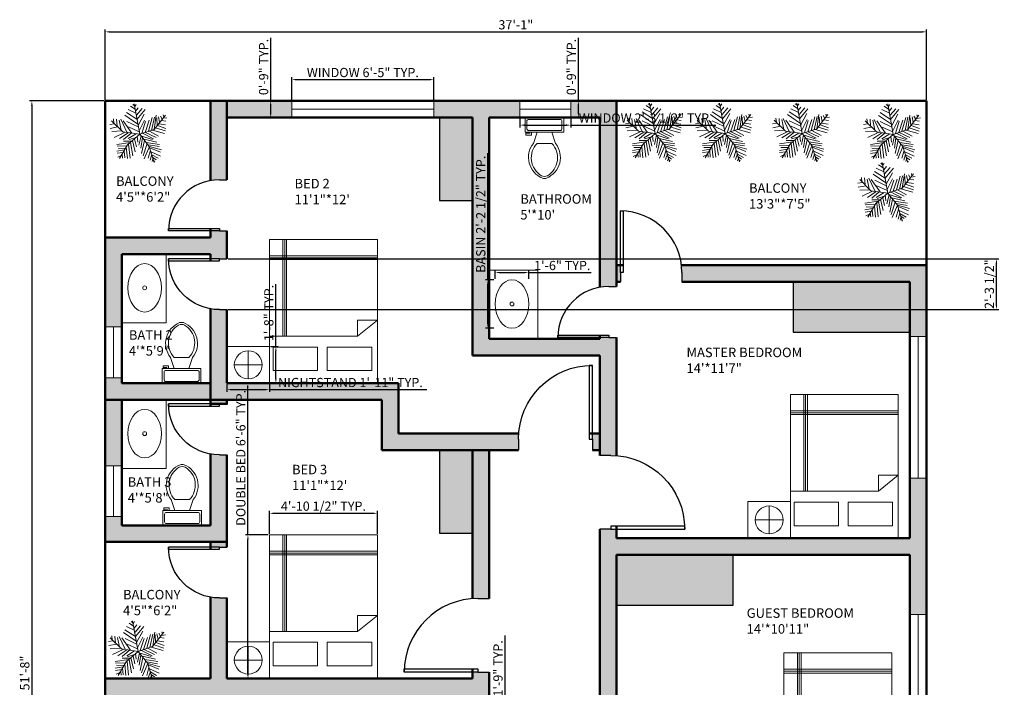
# Model space of a CAD drawing. Units: inches. Extents: x 2091 to 2624, y 1080 to 1790.
# Tile 2 of 2: x 2091 to 2624, y 1429 to 1790. Entities that reach past the tile are written whole.
import ezdxf

# ---------------------------------------------------------------- set-up
doc = ezdxf.new("R2010")
doc.units = ezdxf.units.IN
for name, color, linetype, lineweight in [('A-ANNO-DIMS', 135, 'Continuous', 18), ('A-AREA-IDEN', 135, 'Continuous', 18), ('A-FLOR-CASE', 210, 'Continuous', 25), ('A-FLOR-CASE-PATT', 210, 'Continuous', 13), ('A-FLOR-FIXT', 210, 'Continuous', 18), ('A-WALL-PATT', 190, 'Continuous', 13), ('DOOR', 20, 'Continuous', 25), ('FUR', 210, 'Continuous', 18), ('TREE', 100, 'Continuous', 13), ('WALL', 190, 'Continuous', 50), ('WIND', 10, 'Continuous', 18)]:
    doc.layers.add(name, color=color, linetype=linetype, lineweight=lineweight)
doc.styles.get("Standard").update_dxf_attribs({"font": 'arial.ttf'})
doc.dimstyles.new('ISO-25', dxfattribs={"dimtxt": 5, "dimasz": 2.5, "dimexe": 1.25, "dimexo": 0.625, "dimtad": 1, "dimdec": 0, "dimlunit": 4, "dimtxsty": 'Standard', "dimcen": 2.5, "dimadec": 0, "dimazin": 0, "dimtfac": 1, "dimtdec": 0, "dimtmove": 0, "dimatfit": 3, "dimfxl": 1, "dimarcsym": 0})

# ---------------------------------------------------------------- blocks, each defined once
blk = doc.blocks.new('*U2')
for p, q in [((0, 0), (0, -6)), ((40, 0), (40, -6))]:
    blk.add_line(p, q)
blk.add_lwpolyline([(0, 0), (0, 40), (1.75, 40), (1.75, 0)], close=True)
blk.add_arc((0, 0), 40, 0, 90)
blk = doc.blocks.new('*U4')
for p, q in [((9.5, -6), (9.5, -2)), ((-10, -8.5), (-8, -8.5)), ((-10, -9.5), (-10, -8.5)), ((-7, -9.5), (-10, -9.5)), ((-8, -8.5), (-8, -8)), ((-7, -8), (-7, -9.5)), ((-4, -8), (-6, -14)), ((4, -8), (6, -14)), ((4, -14), (-4, -14))]:
    blk.add_line(p, q)
blk.add_lwpolyline([(10.5, -8), (10.5, 0), (-10.5, 0), (-10.5, -8)], close=True)
for points in [[(-9.5, -2), (-9.5, -6)], [(8.5, -1), (-8.5, -1)], [(-8.5, -7), (8.5, -7)]]:
    blk.add_lwpolyline(points)
for centre, radius, start, end in [((-8.62, -1.88), 0.884, 81.8699, 188.1301), ((8.62, -1.88), 0.884, 351.8699, 98.1301), ((-8.62, -6.12), 0.884, 171.8699, 278.1301), ((8.62, -6.12), 0.884, 261.8699, 8.1301), ((3.52, -21.58), 12.17, 141.4691, 247.9714), ((4.2, -21.82), 11.33, 136.3677, 238.9468), ((-3.52, -21.58), 12.17, 292.0284, 38.5307), ((-4.2, -21.82), 11.33, 301.053, 43.6321), ((0, -27.88), 4, 245.7318, 294.2682), ((0, -29), 4, 254.8605, 285.1395)]:
    blk.add_arc(centre, radius, start, end)
blk = doc.blocks.new('*U6')
for p, q in [((-10.186, 53.64), (-13.084, 55.962)), ((0, 0), (-10.5, 57)), ((-9.099, 51.782), (-6.563, 55.962)), ((-5.114, 28.097), (-24.676, 40.636)), ((-7.288, 39.707), (-21.778, 46.673)), ((-8.737, 47.138), (-17.069, 52.711)), ((-7.65, 43.423), (-2.578, 49.46)), ((-5.839, 35.992), (4.667, 48.067)), ((-5.114, 27.632), (10.463, 46.673)), ((-2.941, 16.486), (8.652, 37.85)), ((-47.498, 19.737), (-55.83, 18.344)), ((-31.5, 4.5), (-52.5, 25.5)), ((-48.585, 21.131), (-49.309, 29.026)), ((-43.513, 28.561), (-42.427, 15.558)), ((-38.442, 26.239), (-34.819, 7.663)), ((-35.544, 28.097), (-24.314, 3.947)), ((-14.533, 2.09), (-30.834, 25.31)), ((-3.665, 19.273), (-27.574, 35.527)), ((-24.314, 23.917), (-2.941, 13.7)), ((-1.129, 6.734), (9.014, 26.704)), ((3.942, 1.625), (11.187, 24.381)), ((10.101, 3.483), (17.708, 26.239)), ((16.259, 5.805), (23.142, 31.348)), ((22.055, 7.198), (27.489, 32.277)), ((27, 9), (48, 36)), ((27.127, 9.056), (31.112, 35.992)), ((31.836, 30.883), (32.561, 16.486)), ((35.096, 32.741), (37.27, 22.524)), ((36.183, 19.737), (48.137, 17.88)), ((38.719, 34.134), (41.979, 28.561)), ((40.53, 25.775), (48.862, 24.846)), ((43.791, 29.954), (51.036, 30.883)), ((44.153, 36.456), (45.239, 32.741)), ((-40.615, 13.7), (-55.105, 10.913)), ((-33.37, 6.269), (-52.207, 5.34)), ((-28.299, 3.483), (-47.86, -5.805)), ((-21.416, 3.018), (-38.079, -8.128)), ((0, 0), (-31.5, 4.5)), ((-15.982, 2.09), (-30.11, -9.521)), ((0, 0), (-22.5, -19.5)), ((-6.563, 1.161), (-21.416, -8.128)), ((-20.691, 13.7), (-1.129, 4.876)), ((0, 0), (27, 9)), ((0, 0), (18, -22.5)), ((6.478, 1.625), (26.04, -8.592)), ((11.187, 3.483), (30.749, -5.805)), ((18.07, 5.805), (35.096, -3.483)), ((24.229, 7.663), (46.688, 1.625)), ((29.662, 12.307), (48.137, 6.269)), ((33.285, 16.486), (48.862, 10.913)), ((-17.431, -15.094), (-42.789, -18.809)), ((-15.257, -12.772), (-30.11, -12.772)), ((-20.691, -18.345), (-17.793, -44.352)), ((-6.563, -5.805), (-19.967, -9.985)), ((-17.069, -15.094), (-12.721, -40.172)), ((-13.446, -11.378), (-8.737, -32.741)), ((-9.461, -8.592), (-6.201, -23.453)), ((-4.752, -3.483), (-3.665, -14.629)), ((2.493, -3.019), (-1.491, -20.202)), ((1.769, -2.555), (24.229, -9.521)), ((5.029, -6.27), (2.131, -25.775)), ((9.014, -11.378), (3.58, -35.992)), ((14.085, -16.951), (6.478, -40.172)), ((7.565, -9.056), (32.198, -14.629)), ((12.274, -15.094), (36.907, -18.809)), ((-28.299, -29.026), (-42.789, -31.348)), ((-24.314, -21.596), (-42.427, -22.06)), ((-30.834, -34.135), (-42.427, -35.528)), ((-26.849, -26.24), (-40.253, -25.775)), ((-22.5, -19.5), (-37.5, -45)), ((-29.023, -30.884), (-27.936, -43.887)), ((-25.038, -23.918), (-22.865, -45.281)), ((18.07, -22.524), (8.289, -45.745)), ((20.244, -30.419), (15.897, -44.816)), ((16.259, -19.738), (36.183, -22.989)), ((18, -22.5), (27, -52.5)), ((18.433, -22.524), (40.53, -29.026)), ((19.157, -25.311), (38.719, -33.206)), ((21.331, -32.741), (39.081, -40.636)), ((-34.457, -39.708), (-40.978, -42.494)), ((-32.646, -36.921), (-31.921, -44.352)), ((22.78, -37.85), (19.519, -48.532)), ((22.78, -38.314), (34.372, -44.816)), ((24.591, -45.745), (23.142, -50.854)), ((24.591, -43.423), (30.749, -47.603)), ((26.764, -49.925), (28.213, -50.854))]:
    blk.add_line(p, q)
blk = doc.blocks.new('*D7')
at = {"layer": 'A-ANNO-DIMS', "color": 0, "lineweight": -2, "transparency": 16777216}
for p, q in [((2137.27, 1746.99), (2137.27, 1785.03)), ((2139.77, 1783.78), (2579.77, 1783.78)), ((2582.27, 1746.99), (2582.27, 1785.03))]:
    blk.add_line(p, q, dxfattribs=at)
at = {"layer": 'A-ANNO-DIMS', "color": 0, "transparency": 16777216}
for points in [[(2139.77, 1784.2), (2139.77, 1783.36), (2137.27, 1783.78)], [(2579.77, 1784.2), (2579.77, 1783.36), (2582.27, 1783.78)]]:
    blk.add_solid(points, dxfattribs=at)
at = {"layer": 'Defpoints', "color": 0, "transparency": 16777216}
for p in [(2582.27, 1783.78), (2137.27, 1746.37), (2582.27, 1746.37)]:
    blk.add_point(p, dxfattribs=at)
at = {"layer": 'A-ANNO-DIMS', "color": 0, "transparency": 16777216, "insert": (2359.77, 1786.96), "char_height": 5, "attachment_point": 5}
blk.add_mtext('37\'-1"', dxfattribs=at)
blk = doc.blocks.new('*D8')
at = {"layer": 'A-ANNO-DIMS', "color": 0, "lineweight": -2, "transparency": 16777216}
for p, q in [((2136.64, 1746.37), (2096.29, 1746.37)), ((2097.54, 1743.87), (2097.54, 1128.87)), ((2136.64, 1126.37), (2096.29, 1126.37))]:
    blk.add_line(p, q, dxfattribs=at)
at = {"layer": 'A-ANNO-DIMS', "color": 0, "transparency": 16777216}
for points in [[(2097.12, 1743.87), (2097.96, 1743.87), (2097.54, 1746.37)], [(2097.12, 1128.87), (2097.96, 1128.87), (2097.54, 1126.37)]]:
    blk.add_solid(points, dxfattribs=at)
at = {"layer": 'Defpoints', "color": 0, "transparency": 16777216}
for p in [(2137.27, 1746.37), (2097.54, 1126.37), (2137.27, 1126.37)]:
    blk.add_point(p, dxfattribs=at)
at = {"layer": 'A-ANNO-DIMS', "color": 0, "transparency": 16777216, "insert": (2094.36, 1436.37), "char_height": 5, "attachment_point": 5, "rotation": 90}
blk.add_mtext('51\'-8"', dxfattribs=at)
blk = doc.blocks.new('BED-DOUBLE')
for p, q in [((7.26, 25.51), (7.26, 77.87)), ((8.26, 25.51), (8.26, 77.87)), ((9.26, 25.51), (9.26, 77.87)), ((0, 69.01), (58.45, 69.01)), ((0, 68.01), (58.45, 68.01)), ((0, 67.01), (58.45, 67.01)), ((47.64, 25.51), (47.64, 34.16)), ((47.64, 34.16), (58.45, 34.16)), ((58.45, 34.16), (47.64, 25.51)), ((0, 25.51), (47.64, 25.51))]:
    blk.add_line(p, q)
for points in [[(0, 0), (58.45, 0), (58.45, 77.87), (0, 77.87)], [(1.98, 6.84), (26.02, 6.84), (26.02, 19.63), (1.98, 19.63)], [(31.32, 6.84), (55.36, 6.84), (55.36, 19.63), (31.32, 19.63)]]:
    blk.add_lwpolyline(points, close=True)
blk = doc.blocks.new('NIGHTSTAND-LAMP')
for p, q in [((11.52, 2.41), (11.52, 17.54)), ((3.95, 9.98), (19.08, 9.98)), ((11.52, 9.98), (11.52, 2.41))]:
    blk.add_line(p, q)
blk.add_lwpolyline([(23.03, 0), (0, 0), (0, 19.96), (23.03, 19.96)], close=True)
blk.add_circle((11.52, 9.98), 7.56)
blk = doc.blocks.new('LAVATORY-BASIN')
blk.add_circle((9.11, 13.13), 1.04)
blk.add_ellipse((9.11, 13.13), major_axis=(0, 13.13), ratio=0.694107)
blk = doc.blocks.new('WIN-76_81')
blk.add_line((0, 4.5), (76.81, 4.5))
blk.add_lwpolyline([(0, 0), (76.81, 0), (76.81, 9), (0, 9)], close=True)
blk = doc.blocks.new('WIN-27_52')
blk.add_line((0, 4.5), (27.52, 4.5))
blk.add_lwpolyline([(0, 0), (27.52, 0), (27.52, 9), (0, 9)], close=True)
blk = doc.blocks.new('*D16')
at = {"layer": 'A-ANNO-DIMS', "color": 0, "lineweight": -2, "transparency": 16777216}
for p, q in [((2362.02, 1736.74), (2362.02, 1731.99)), ((2389.54, 1736.74), (2389.54, 1731.99)), ((2364.52, 1733.24), (2387.04, 1733.24)), ((2389.54, 1733.24), (2468.21, 1733.24))]:
    blk.add_line(p, q, dxfattribs=at)
at = {"layer": 'A-ANNO-DIMS', "color": 0, "transparency": 16777216}
for points in [[(2364.52, 1733.66), (2364.52, 1732.82), (2362.02, 1733.24)], [(2387.04, 1733.66), (2387.04, 1732.82), (2389.54, 1733.24)]]:
    blk.add_solid(points, dxfattribs=at)
at = {"layer": 'Defpoints', "color": 0, "transparency": 16777216}
for p in [(2362.02, 1737.37), (2389.54, 1737.37), (2389.54, 1733.24)]:
    blk.add_point(p, dxfattribs=at)
at = {"layer": 'A-ANNO-DIMS', "color": 0, "transparency": 16777216, "insert": (2430.12, 1736.45), "char_height": 5, "attachment_point": 5}
blk.add_mtext('WINDOW 2\'-3 1/2" TYP.', dxfattribs=at)
blk = doc.blocks.new('*D17')
at = {"layer": 'A-ANNO-DIMS', "color": 0, "lineweight": -2, "transparency": 16777216}
for p, q in [((2393.66, 1746.37), (2393.66, 1780.59)), ((2390.16, 1746.37), (2394.91, 1746.37)), ((2393.66, 1739.87), (2393.66, 1743.87)), ((2390.16, 1737.37), (2394.91, 1737.37))]:
    blk.add_line(p, q, dxfattribs=at)
at = {"layer": 'A-ANNO-DIMS', "color": 0, "transparency": 16777216}
for points in [[(2393.25, 1743.87), (2394.08, 1743.87), (2393.66, 1746.37)], [(2393.25, 1739.87), (2394.08, 1739.87), (2393.66, 1737.37)]]:
    blk.add_solid(points, dxfattribs=at)
at = {"layer": 'Defpoints', "color": 0, "transparency": 16777216}
for p in [(2389.54, 1746.37), (2393.66, 1746.37), (2389.54, 1737.37)]:
    blk.add_point(p, dxfattribs=at)
at = {"layer": 'A-ANNO-DIMS', "color": 0, "transparency": 16777216, "insert": (2390.49, 1764.73), "char_height": 5, "attachment_point": 5, "rotation": 90}
blk.add_mtext('0\'-9" TYP.', dxfattribs=at)
blk = doc.blocks.new('*D18')
at = {"layer": 'A-ANNO-DIMS', "color": 0, "lineweight": -2, "transparency": 16777216}
for p, q in [((2238.46, 1746.99), (2238.46, 1759.14)), ((2240.96, 1757.89), (2312.77, 1757.89)), ((2315.27, 1746.99), (2315.27, 1759.14))]:
    blk.add_line(p, q, dxfattribs=at)
at = {"layer": 'A-ANNO-DIMS', "color": 0, "transparency": 16777216}
for points in [[(2240.96, 1758.31), (2240.96, 1757.47), (2238.46, 1757.89)], [(2312.77, 1758.31), (2312.77, 1757.47), (2315.27, 1757.89)]]:
    blk.add_solid(points, dxfattribs=at)
at = {"layer": 'Defpoints', "color": 0, "transparency": 16777216}
for p in [(2315.27, 1757.89), (2238.46, 1746.37), (2315.27, 1746.37)]:
    blk.add_point(p, dxfattribs=at)
at = {"layer": 'A-ANNO-DIMS', "color": 0, "transparency": 16777216, "insert": (2276.87, 1761.1), "char_height": 5, "attachment_point": 5}
blk.add_mtext('WINDOW 6\'-5" TYP.', dxfattribs=at)
blk = doc.blocks.new('*D19')
at = {"layer": 'A-ANNO-DIMS', "color": 0, "lineweight": -2, "transparency": 16777216}
for p, q in [((2226.94, 1746.37), (2226.94, 1780.59)), ((2237.84, 1746.37), (2225.69, 1746.37)), ((2226.94, 1739.87), (2226.94, 1743.87)), ((2237.84, 1737.37), (2225.69, 1737.37))]:
    blk.add_line(p, q, dxfattribs=at)
at = {"layer": 'A-ANNO-DIMS', "color": 0, "transparency": 16777216}
for points in [[(2226.52, 1743.87), (2227.36, 1743.87), (2226.94, 1746.37)], [(2226.52, 1739.87), (2227.36, 1739.87), (2226.94, 1737.37)]]:
    blk.add_solid(points, dxfattribs=at)
at = {"layer": 'Defpoints', "color": 0, "transparency": 16777216}
for p in [(2226.94, 1746.37), (2238.46, 1746.37), (2238.46, 1737.37)]:
    blk.add_point(p, dxfattribs=at)
at = {"layer": 'A-ANNO-DIMS', "color": 0, "transparency": 16777216, "insert": (2223.76, 1764.73), "char_height": 5, "attachment_point": 5, "rotation": 90}
blk.add_mtext('0\'-9" TYP.', dxfattribs=at)
blk = doc.blocks.new('*D20')
at = {"layer": 'A-ANNO-DIMS', "color": 0, "lineweight": -2, "transparency": 16777216}
for p, q in [((2214.62, 1511.24), (2214.62, 1592.18)), ((2225.67, 1511.24), (2213.37, 1511.24)), ((2214.62, 1435.87), (2214.62, 1508.74)), ((2225.67, 1433.37), (2213.37, 1433.37))]:
    blk.add_line(p, q, dxfattribs=at)
at = {"layer": 'A-ANNO-DIMS', "color": 0, "transparency": 16777216}
for points in [[(2214.2, 1508.74), (2215.04, 1508.74), (2214.62, 1511.24)], [(2214.2, 1435.87), (2215.04, 1435.87), (2214.62, 1433.37)]]:
    blk.add_solid(points, dxfattribs=at)
at = {"layer": 'Defpoints', "color": 0, "transparency": 16777216}
for p in [(2214.62, 1511.24), (2226.3, 1511.24), (2226.3, 1433.37)]:
    blk.add_point(p, dxfattribs=at)
at = {"layer": 'A-ANNO-DIMS', "color": 0, "transparency": 16777216, "insert": (2211.41, 1552.96), "char_height": 5, "attachment_point": 5, "rotation": 90}
blk.add_mtext('DOUBLE BED 6\'-6" TYP.', dxfattribs=at)
blk = doc.blocks.new('*D21')
at = {"layer": 'A-ANNO-DIMS', "color": 0, "lineweight": -2, "transparency": 16777216}
for p, q in [((2226.3, 1511.86), (2226.3, 1524.17)), ((2228.8, 1522.92), (2282.25, 1522.92)), ((2284.75, 1511.86), (2284.75, 1524.17))]:
    blk.add_line(p, q, dxfattribs=at)
at = {"layer": 'A-ANNO-DIMS', "color": 0, "transparency": 16777216}
for points in [[(2228.8, 1523.33), (2228.8, 1522.5), (2226.3, 1522.92)], [(2282.25, 1523.33), (2282.25, 1522.5), (2284.75, 1522.92)]]:
    blk.add_solid(points, dxfattribs=at)
at = {"layer": 'Defpoints', "color": 0, "transparency": 16777216}
for p in [(2284.75, 1522.92), (2226.3, 1511.24), (2284.75, 1511.24)]:
    blk.add_point(p, dxfattribs=at)
at = {"layer": 'A-ANNO-DIMS', "color": 0, "transparency": 16777216, "insert": (2255.52, 1526.13), "char_height": 5, "attachment_point": 5}
blk.add_mtext('4\'-10 1/2" TYP.', dxfattribs=at)
blk = doc.blocks.new('*D22')
at = {"layer": 'A-ANNO-DIMS', "color": 0, "lineweight": -2, "transparency": 16777216}
for p, q in [((2203.27, 1592.74), (2203.27, 1588.66)), ((2205.77, 1589.91), (2223.8, 1589.91)), ((2226.3, 1592.74), (2226.3, 1588.66)), ((2226.3, 1589.91), (2311.51, 1589.91))]:
    blk.add_line(p, q, dxfattribs=at)
at = {"layer": 'A-ANNO-DIMS', "color": 0, "transparency": 16777216}
for points in [[(2205.77, 1590.33), (2205.77, 1589.5), (2203.27, 1589.91)], [(2223.8, 1590.33), (2223.8, 1589.5), (2226.3, 1589.91)]]:
    blk.add_solid(points, dxfattribs=at)
at = {"layer": 'Defpoints', "color": 0, "transparency": 16777216}
for p in [(2203.27, 1593.37), (2226.3, 1593.37), (2226.3, 1589.91)]:
    blk.add_point(p, dxfattribs=at)
at = {"layer": 'A-ANNO-DIMS', "color": 0, "transparency": 16777216, "insert": (2270.16, 1593.12), "char_height": 5, "attachment_point": 5}
blk.add_mtext('NIGHTSTAND 1\'-11" TYP.', dxfattribs=at)
blk = doc.blocks.new('*D23')
at = {"layer": 'A-ANNO-DIMS', "color": 0, "lineweight": -2, "transparency": 16777216}
for p, q in [((2229.75, 1613.32), (2229.75, 1647.08)), ((2226.92, 1613.32), (2231, 1613.32)), ((2229.75, 1595.87), (2229.75, 1610.82)), ((2226.92, 1593.37), (2231, 1593.37))]:
    blk.add_line(p, q, dxfattribs=at)
at = {"layer": 'A-ANNO-DIMS', "color": 0, "transparency": 16777216}
for points in [[(2229.34, 1610.82), (2230.17, 1610.82), (2229.75, 1613.32)], [(2229.34, 1595.87), (2230.17, 1595.87), (2229.75, 1593.37)]]:
    blk.add_solid(points, dxfattribs=at)
at = {"layer": 'Defpoints', "color": 0, "transparency": 16777216}
for p in [(2226.3, 1613.32), (2229.75, 1613.32), (2226.3, 1593.37)]:
    blk.add_point(p, dxfattribs=at)
at = {"layer": 'A-ANNO-DIMS', "color": 0, "transparency": 16777216, "insert": (2226.58, 1631.45), "char_height": 5, "attachment_point": 5, "rotation": 90}
blk.add_mtext('1\'-8" TYP.', dxfattribs=at)
blk = doc.blocks.new('*D24')
at = {"layer": 'A-ANNO-DIMS', "color": 0, "lineweight": -2, "transparency": 16777216}
for p, q in [((2344.63, 1649.42), (2344.63, 1717.98)), ((2347.94, 1649.42), (2343.38, 1649.42)), ((2344.63, 1625.67), (2344.63, 1646.92)), ((2347.94, 1623.17), (2343.38, 1623.17))]:
    blk.add_line(p, q, dxfattribs=at)
at = {"layer": 'A-ANNO-DIMS', "color": 0, "transparency": 16777216}
for points in [[(2344.21, 1646.92), (2345.05, 1646.92), (2344.63, 1649.42)], [(2344.21, 1625.67), (2345.05, 1625.67), (2344.63, 1623.17)]]:
    blk.add_solid(points, dxfattribs=at)
at = {"layer": 'Defpoints', "color": 0, "transparency": 16777216}
for p in [(2344.63, 1649.42), (2348.57, 1649.42), (2348.57, 1623.17)]:
    blk.add_point(p, dxfattribs=at)
at = {"layer": 'A-ANNO-DIMS', "color": 0, "transparency": 16777216, "insert": (2341.42, 1684.95), "char_height": 5, "attachment_point": 5, "rotation": 90}
blk.add_mtext('BASIN 2\'-2 1/2" TYP.', dxfattribs=at)
blk = doc.blocks.new('*D25')
at = {"layer": 'A-ANNO-DIMS', "color": 0, "lineweight": -2, "transparency": 16777216}
for p, q in [((2348.57, 1650.04), (2348.57, 1654.61)), ((2366.79, 1650.04), (2366.79, 1654.61)), ((2351.07, 1653.36), (2364.29, 1653.36)), ((2366.79, 1653.36), (2400.55, 1653.36))]:
    blk.add_line(p, q, dxfattribs=at)
at = {"layer": 'A-ANNO-DIMS', "color": 0, "transparency": 16777216}
for points in [[(2351.07, 1653.77), (2351.07, 1652.94), (2348.57, 1653.36)], [(2364.29, 1653.77), (2364.29, 1652.94), (2366.79, 1653.36)]]:
    blk.add_solid(points, dxfattribs=at)
at = {"layer": 'Defpoints', "color": 0, "transparency": 16777216}
for p in [(2348.57, 1649.42), (2366.79, 1653.36), (2366.79, 1649.42)]:
    blk.add_point(p, dxfattribs=at)
at = {"layer": 'A-ANNO-DIMS', "color": 0, "transparency": 16777216, "insert": (2384.92, 1656.53), "char_height": 5, "attachment_point": 5}
blk.add_mtext('1\'-6" TYP.', dxfattribs=at)
blk = doc.blocks.new('*D26')
at = {"layer": 'A-ANNO-DIMS', "color": 0, "lineweight": -2, "transparency": 16777216}
for p, q in [((2353.97, 1372.58), (2353.97, 1456.62)), ((2351.48, 1372.58), (2355.22, 1372.58)), ((2353.97, 1354.31), (2353.97, 1370.08)), ((2351.48, 1351.81), (2355.22, 1351.81))]:
    blk.add_line(p, q, dxfattribs=at)
at = {"layer": 'A-ANNO-DIMS', "color": 0, "transparency": 16777216}
for points in [[(2353.56, 1370.08), (2354.39, 1370.08), (2353.97, 1372.58)], [(2353.56, 1354.31), (2354.39, 1354.31), (2353.97, 1351.81)]]:
    blk.add_solid(points, dxfattribs=at)
at = {"layer": 'Defpoints', "color": 0, "transparency": 16777216}
for p in [(2350.86, 1372.58), (2353.97, 1372.58), (2350.86, 1351.81)]:
    blk.add_point(p, dxfattribs=at)
at = {"layer": 'A-ANNO-DIMS', "color": 0, "transparency": 16777216, "insert": (2350.76, 1415.85), "char_height": 5, "attachment_point": 5, "rotation": 90}
blk.add_mtext('DINING CHAIR 1\'-9" TYP.', dxfattribs=at)
blk = doc.blocks.new('*D31')
at = {"layer": 'A-ANNO-DIMS', "color": 0, "lineweight": -2, "transparency": 16777216}
for p, q in [((2203.89, 1660.87), (2621.44, 1660.87)), ((2620.19, 1635.78), (2620.19, 1658.37)), ((2203.89, 1633.28), (2621.44, 1633.28))]:
    blk.add_line(p, q, dxfattribs=at)
at = {"layer": 'A-ANNO-DIMS', "color": 0, "transparency": 16777216}
for points in [[(2619.77, 1658.37), (2620.6, 1658.37), (2620.19, 1660.87)], [(2619.77, 1635.78), (2620.6, 1635.78), (2620.19, 1633.28)]]:
    blk.add_solid(points, dxfattribs=at)
at = {"layer": 'Defpoints', "color": 0, "transparency": 16777216}
for p in [(2203.27, 1660.87), (2620.19, 1660.87), (2203.27, 1633.28)]:
    blk.add_point(p, dxfattribs=at)
at = {"layer": 'A-ANNO-DIMS', "color": 0, "transparency": 16777216, "insert": (2616.97, 1647.08), "char_height": 5, "attachment_point": 5, "rotation": 90}
blk.add_mtext('2\'-3 1/2"', dxfattribs=at)

msp = doc.modelspace()

# ---------------------------------------------------------------- hatches: boundary and pattern name
at = {"layer": 'A-FLOR-CASE-PATT'}
h = msp.add_hatch(color=256, dxfattribs=at)
h.dxf.hatch_style = 1
h.paths.add_polyline_path([(2336.27, 1737.37), (2318.34, 1737.37), (2318.34, 1692.36), (2336.27, 1692.36)])
h.paths.add_polyline_path([(2573.27, 1648.37), (2510.08, 1648.37), (2510.08, 1621.07), (2573.27, 1621.07)])
h.paths.add_polyline_path([(2336.27, 1557.08), (2318.34, 1557.08), (2318.34, 1512.08), (2336.27, 1512.08)])
h.paths.add_polyline_path([(2477.45, 1500.37), (2414.27, 1500.37), (2414.27, 1473.07), (2477.45, 1473.07)])
at = {"layer": 'A-WALL-PATT'}
h = msp.add_hatch(color=256, dxfattribs=at)
h.dxf.hatch_style = 1
h.paths.add_polyline_path([(2203.27, 1737.37), (2203.27, 1746.37), (2194.27, 1746.37), (2194.27, 1703.2, -0.044322), (2199.13, 1703.63), (2203.27, 1703.63)])
h.paths.add_polyline_path([(2238.46, 1746.37), (2203.27, 1746.37), (2203.27, 1737.37), (2238.46, 1737.37)])
h.paths.add_polyline_path([(2194.27, 1593.37), (2146.27, 1593.37), (2146.27, 1596.35), (2137.27, 1596.35), (2137.27, 1584.37), (2194.27, 1584.37)])
h.paths.add_polyline_path([(2146.27, 1584.37), (2137.27, 1584.37), (2137.27, 1548.65), (2146.27, 1548.65)])
h.paths.add_polyline_path([(2203.27, 1554.64), (2199.13, 1554.64, -0.044322), (2194.27, 1555.07), (2194.27, 1516.37), (2146.27, 1516.37), (2146.27, 1521.14), (2137.27, 1521.14), (2137.27, 1507.37), (2203.27, 1507.37)])
h.paths.add_polyline_path([(2345.27, 1436.81), (2339.27, 1436.81), (2336.27, 1436.81), (2336.27, 1433.37), (2203.27, 1433.37), (2203.27, 1453.32), (2203.27, 1477.02), (2199.13, 1477.02, -0.044322), (2194.27, 1477.45), (2194.27, 1433.37), (2137.27, 1433.37), (2137.27, 1424.37), (2137.27, 1416.56), (2146.27, 1416.56), (2146.27, 1424.37), (2242.27, 1424.37), (2345.27, 1424.37)])
h.paths.add_polyline_path([(2345.27, 1557.08), (2336.27, 1557.08), (2336.27, 1512.08), (2336.27, 1476.7, -0.01877), (2339.27, 1476.81), (2345.27, 1476.81)])
h.paths.add_polyline_path([(2146.27, 1356.3), (2137.27, 1356.3), (2137.27, 1339.9), (2146.27, 1339.9)])
h.paths.add_polyline_path([(2251.27, 1307.84), (2245.27, 1307.84), (2242.27, 1307.84), (2242.27, 1304.37), (2146.27, 1304.37), (2146.27, 1312.38), (2137.27, 1312.38), (2137.27, 1295.37), (2137.27, 1280.09), (2146.27, 1280.09), (2146.27, 1295.37), (2206.27, 1295.37), (2206.27, 1279.55, -0.044322), (2211.13, 1279.98), (2215.27, 1279.98), (2215.27, 1295.37), (2251.27, 1295.37)])
h.paths.add_polyline_path([(2251.27, 1424.37), (2242.27, 1424.37), (2242.27, 1347.73, -0.01877), (2245.27, 1347.84), (2251.27, 1347.84)])
h.paths.add_polyline_path([(2146.27, 1240.37), (2169.1, 1240.37), (2192.27, 1240.37), (2192.27, 1238.44), (2197.13, 1238.44), (2201.27, 1238.44), (2201.27, 1240.37), (2215.27, 1240.37), (2215.27, 1252.39), (2211.13, 1252.39), (2206.27, 1252.39), (2206.27, 1249.37), (2146.27, 1249.37), (2146.27, 1252.57), (2137.27, 1252.57), (2137.27, 1240.37), (2137.27, 1208.01), (2146.27, 1208.01)])
h.paths.add_polyline_path([(2146.27, 1180.49), (2137.27, 1180.49), (2137.27, 1126.37), (2168.5, 1126.37), (2168.5, 1135.37), (2146.27, 1135.37)])
h.paths.add_polyline_path([(2316.01, 1135.37), (2228.53, 1135.37), (2228.53, 1126.37), (2316.01, 1126.37)])
h.paths.add_polyline_path([(2582.27, 1143.15), (2573.27, 1143.15), (2573.27, 1135.37), (2531.27, 1135.37), (2377.62, 1135.37), (2377.62, 1126.37), (2582.27, 1126.37)])
h.paths.add_polyline_path([(2582.27, 1277.86), (2573.27, 1277.86), (2573.27, 1240.37), (2429.27, 1240.37), (2429.27, 1264.37), (2429.27, 1315.33, -0.01877), (2426.27, 1315.22), (2420.27, 1315.22), (2420.27, 1240.37), (2390.27, 1240.37), (2390.27, 1228.4, -0.01877), (2393.27, 1228.51), (2399.27, 1228.51), (2399.27, 1231.37), (2420.27, 1231.37), (2573.27, 1231.37), (2573.27, 1219.96), (2582.27, 1219.96), (2582.27, 1231.37)])
h.paths.add_polyline_path([(2582.27, 1391.21), (2573.27, 1391.21), (2573.27, 1369.37), (2414.27, 1369.37), (2414.27, 1374.96), (2411.27, 1374.96), (2405.27, 1374.96), (2405.27, 1360.37), (2573.27, 1360.37), (2573.27, 1333.61), (2582.27, 1333.61), (2582.27, 1360.37)])
h.paths.add_polyline_path([(2582.27, 1541.89), (2573.27, 1541.89), (2573.27, 1509.37), (2414.27, 1509.37), (2414.27, 1514.26), (2411.27, 1514.26), (2405.27, 1514.26), (2405.27, 1500.37), (2405.27, 1414.96), (2411.27, 1414.96, -0.01877), (2414.27, 1414.85), (2414.27, 1500.37), (2477.45, 1500.37), (2573.27, 1500.37), (2573.27, 1468.02), (2582.27, 1468.02), (2582.27, 1500.37)])
h.paths.add_polyline_path([(2236.44, 1532.62), (2267.09, 1532.62), (2267.09, 1551.82), (2236.44, 1551.82)], flags=9)
h.paths.add_polyline_path([(2148.33, 1605.52), (2176.06, 1605.52), (2176.06, 1624.71), (2148.33, 1624.71)], flags=9)
h.paths.add_polyline_path([(2360.41, 1679.17), (2404.5, 1679.17), (2404.5, 1698.37), (2360.41, 1698.37)], flags=9)
h.paths.add_polyline_path([(2484.05, 1685.08), (2521.22, 1685.08), (2521.22, 1704.27), (2484.05, 1704.27)], flags=9)
h.paths.add_polyline_path([(2450.18, 1596.03), (2522.07, 1596.03), (2522.07, 1615.22), (2450.18, 1615.22)], flags=9)
h.paths.add_polyline_path([(2482.78, 1454.78), (2549.63, 1454.78), (2549.63, 1473.97), (2482.78, 1473.97)], flags=25)
h.paths.add_polyline_path([(2476.32, 1294.17), (2510.69, 1294.17), (2510.69, 1313.36), (2476.32, 1313.36)], flags=25)
h.paths.add_polyline_path([(2281, 1265.16), (2341.07, 1265.16), (2341.07, 1284.35), (2281, 1284.35)], flags=9)
h.paths.add_polyline_path([(2151.29, 1184.31), (2187.39, 1184.31), (2187.39, 1212.17), (2151.29, 1212.17)], flags=9)
h.paths.add_polyline_path([(2152.56, 1259.62), (2188.66, 1259.62), (2188.66, 1287.47), (2152.56, 1287.47)], flags=9)
h.paths.add_polyline_path([(2171.26, 1375.61), (2227.73, 1375.61), (2227.73, 1394.8), (2171.26, 1394.8)], flags=9)
h.paths.add_polyline_path([(2145.13, 1464.78), (2182.05, 1464.78), (2182.05, 1483.97), (2145.13, 1483.97)], flags=9)
h.paths.add_polyline_path([(2147.67, 1525.88), (2175.4, 1525.88), (2175.4, 1545.07), (2147.67, 1545.07)], flags=25)
h.paths.add_polyline_path([(2237.82, 1687.57), (2268.47, 1687.57), (2268.47, 1706.76), (2237.82, 1706.76)], flags=9)
h.paths.add_polyline_path([(2141.34, 1688.84), (2178.25, 1688.84), (2178.25, 1708.04), (2141.34, 1708.04)], flags=9)
h = msp.add_hatch(color=256, dxfattribs=at)
h.dxf.hatch_style = 1
h.paths.add_polyline_path([(2203.27, 1676.04), (2199.13, 1676.04), (2194.27, 1676.04), (2194.27, 1672.37), (2141.27, 1672.37), (2137.27, 1672.37), (2137.27, 1663.37), (2137.27, 1623.87), (2146.27, 1623.87), (2146.27, 1663.37), (2170.31, 1663.37), (2194.27, 1663.37), (2194.27, 1660.87), (2199.13, 1660.87), (2203.27, 1660.87)])
h.paths.add_polyline_path([(2203.27, 1613.32), (2203.27, 1633.28), (2199.13, 1633.28, -0.044322), (2194.27, 1633.71), (2194.27, 1584.37), (2287.2, 1584.37), (2287.2, 1557.08), (2336.27, 1557.08), (2361.22, 1557.08), (2361.22, 1563.08, -0.01877), (2361.33, 1566.08), (2345.27, 1566.08), (2296.2, 1566.08), (2296.2, 1593.37), (2203.27, 1593.37)])
h.paths.add_polyline_path([(2345.27, 1737.37), (2362.02, 1737.37), (2362.02, 1746.37), (2345.27, 1746.37), (2315.27, 1746.37), (2315.27, 1737.37), (2336.27, 1737.37), (2336.27, 1608.37), (2405.27, 1608.37), (2405.27, 1554.26), (2411.27, 1554.26, -0.01877), (2414.27, 1554.15), (2414.27, 1618.21), (2410.13, 1618.21), (2405.27, 1618.21), (2405.27, 1617.37), (2345.27, 1617.37), (2345.27, 1654.59)])
h.paths.add_polyline_path([(2582.27, 1657.37), (2449.52, 1657.37, -0.030027), (2449.76, 1653.37), (2449.76, 1648.37), (2573.27, 1648.37), (2573.27, 1621.07), (2573.27, 1618.7), (2582.27, 1618.7)])
h.paths.add_polyline_path([(2414.27, 1746.37), (2389.54, 1746.37), (2389.54, 1737.37), (2405.27, 1737.37), (2405.27, 1645.37, -0.044322), (2410.13, 1645.8), (2414.27, 1645.8)], flags=17)
h.paths.add_polyline_path([(2405.27, 1566.08), (2401.22, 1566.08), (2401.22, 1563.08), (2401.22, 1557.08), (2405.27, 1557.08)], flags=17)
h = msp.add_hatch(color=256, dxfattribs=at)
h.dxf.hatch_style = 1
h.paths.add_polyline_path([(2203.27, 1584.37), (2194.27, 1584.37), (2194.27, 1582.22), (2199.13, 1582.22), (2203.27, 1582.22)])
h.paths.add_polyline_path([(2416.4, 1653.37), (2416.4, 1657.37), (2414.27, 1657.37), (2414.27, 1648.37), (2416.4, 1648.37)])
h = msp.add_hatch(color=256, dxfattribs=at)
h.dxf.hatch_style = 1
h.paths.add_polyline_path([(2399.27, 1188.51), (2393.27, 1188.51), (2390.27, 1188.51), (2390.27, 1135.37), (2399.27, 1135.37)])
h.paths.add_polyline_path([(2429.27, 1360.37), (2420.27, 1360.37), (2420.27, 1355.22), (2426.27, 1355.22), (2429.27, 1355.22)])
h.paths.add_polyline_path([(2198.16, 1352.23), (2184.99, 1352.23), (2146.27, 1352.23), (2146.27, 1347.73), (2184.99, 1347.73), (2198.16, 1347.73)])
h.paths.add_polyline_path([(2203.27, 1507.37), (2194.27, 1507.37), (2194.27, 1504.61), (2199.13, 1504.61), (2203.27, 1504.61)])

# ---------------------------------------------------------------- linework, layer by layer
at = {"layer": 'A-FLOR-CASE'}
for points in [[(2336.27, 1737.37), (2318.34, 1737.37), (2318.34, 1692.36), (2336.27, 1692.36)], [(2573.27, 1648.37), (2510.08, 1648.37), (2510.08, 1621.07), (2573.27, 1621.07)], [(2336.27, 1557.08), (2318.34, 1557.08), (2318.34, 1512.08), (2336.27, 1512.08)], [(2477.45, 1500.37), (2414.27, 1500.37), (2414.27, 1473.07), (2477.45, 1473.07)]]:
    msp.add_lwpolyline(points, close=True, dxfattribs=at)
at = {"layer": 'A-FLOR-FIXT'}
for points in [[(2146.27, 1626.15), (2170.31, 1626.15), (2170.31, 1663.37), (2146.27, 1663.37)], [(2345.27, 1617.37), (2371.7, 1617.37), (2371.7, 1654.59), (2345.27, 1654.59)], [(2146.27, 1547.15), (2170.31, 1547.15), (2170.31, 1584.37), (2146.27, 1584.37)]]:
    msp.add_lwpolyline(points, close=True, dxfattribs=at)
at = {"layer": 'WALL'}
for p, q in [((2137.27, 1746.37), (2203.27, 1746.37)), ((2137.27, 1746.37), (2137.27, 1663.37)), ((2194.27, 1746.37), (2194.27, 1703.2)), ((2203.27, 1746.37), (2203.27, 1703.63)), ((2203.27, 1746.37), (2345.27, 1746.37)), ((2345.27, 1746.37), (2414.27, 1746.37)), ((2414.27, 1746.37), (2414.27, 1645.8)), ((2414.27, 1746.37), (2582.27, 1746.37)), ((2582.27, 1746.37), (2582.27, 1657.37)), ((2194.27, 1737.37), (2194.27, 1703.2)), ((2203.27, 1737.37), (2336.27, 1737.37)), ((2203.27, 1737.37), (2203.27, 1703.63)), ((2336.27, 1608.37), (2336.27, 1737.37)), ((2345.27, 1617.37), (2345.27, 1737.37)), ((2345.27, 1737.37), (2405.27, 1737.37)), ((2405.27, 1737.37), (2405.27, 1645.37)), ((2194.27, 1677.25), (2194.27, 1672.37)), ((2194.27, 1677.25), (2194.27, 1672.37)), ((2203.27, 1676.04), (2203.27, 1660.87)), ((2203.27, 1676.04), (2203.27, 1663.37)), ((2141.27, 1672.37), (2137.27, 1672.37)), ((2194.27, 1672.37), (2141.27, 1672.37)), ((2137.27, 1663.37), (2137.27, 1584.37)), ((2194.27, 1663.37), (2146.27, 1663.37)), ((2194.27, 1663.37), (2146.27, 1663.37)), ((2194.27, 1663.37), (2146.27, 1663.37)), ((2146.27, 1663.37), (2146.27, 1593.37)), ((2194.27, 1663.37), (2194.27, 1659.66)), ((2417.86, 1657.37), (2414.27, 1657.37)), ((2582.27, 1657.37), (2449.52, 1657.37)), ((2582.27, 1657.37), (2582.27, 1500.37)), ((2405.27, 1648.37), (2405.27, 1645.37)), ((2414.27, 1648.37), (2414.27, 1645.8)), ((2416.4, 1648.37), (2414.27, 1648.37)), ((2573.27, 1648.37), (2449.76, 1648.37)), ((2573.27, 1648.37), (2573.27, 1509.37)), ((2194.27, 1633.71), (2194.27, 1584.37)), ((2203.27, 1633.28), (2203.27, 1593.37)), ((2405.27, 1617.37), (2345.27, 1617.37)), ((2405.27, 1619.42), (2405.27, 1617.37)), ((2405.27, 1619.42), (2405.27, 1617.37)), ((2414.27, 1618.21), (2414.27, 1554.15)), ((2414.27, 1618.21), (2414.27, 1608.37)), ((2405.27, 1608.37), (2336.27, 1608.37)), ((2405.27, 1608.37), (2405.27, 1554.26)), ((2146.27, 1593.37), (2194.27, 1593.37)), ((2203.27, 1593.37), (2296.2, 1593.37)), ((2296.2, 1593.37), (2296.2, 1566.08)), ((2137.27, 1585.37), (2137.27, 1517.37)), ((2137.27, 1584.37), (2194.27, 1584.37)), ((2137.27, 1584.37), (2137.27, 1507.37)), ((2146.27, 1584.37), (2146.27, 1516.37)), ((2194.27, 1584.37), (2287.2, 1584.37)), ((2194.27, 1581.02), (2194.27, 1584.37)), ((2203.27, 1584.37), (2203.27, 1582.22)), ((2203.27, 1582.22), (2203.27, 1584.37)), ((2287.2, 1584.37), (2287.2, 1557.08)), ((2296.2, 1566.08), (2345.27, 1566.08)), ((2345.27, 1566.08), (2361.33, 1566.08)), ((2399.47, 1566.08), (2405.27, 1566.08)), ((2194.27, 1516.37), (2194.27, 1555.07)), ((2203.27, 1507.37), (2203.27, 1554.64)), ((2203.27, 1554.64), (2203.27, 1504.61)), ((2287.2, 1557.08), (2336.27, 1557.08)), ((2336.27, 1557.08), (2361.22, 1557.08)), ((2336.27, 1476.7), (2336.27, 1557.08)), ((2345.27, 1476.81), (2345.27, 1557.08)), ((2401.22, 1557.08), (2405.27, 1557.08)), ((2137.27, 1424.37), (2137.27, 1517.37)), ((2146.27, 1516.37), (2194.27, 1516.37)), ((2414.27, 1516.01), (2414.27, 1509.37)), ((2405.27, 1514.26), (2405.27, 1500.37)), ((2137.27, 1507.37), (2203.27, 1507.37)), ((2194.27, 1507.37), (2194.27, 1503.4)), ((2203.27, 1507.37), (2203.27, 1504.61)), ((2414.27, 1509.37), (2573.27, 1509.37)), ((2405.27, 1500.37), (2405.27, 1414.96)), ((2414.27, 1500.37), (2573.27, 1500.37)), ((2414.27, 1500.37), (2414.27, 1414.85)), ((2573.27, 1500.37), (2573.27, 1369.37)), ((2582.27, 1500.37), (2582.27, 1360.37)), ((2194.27, 1477.45), (2194.27, 1433.37)), ((2203.27, 1477.02), (2203.27, 1440.37)), ((2203.27, 1477.02), (2203.27, 1433.37)), ((2336.27, 1433.37), (2336.27, 1438.56)), ((2345.27, 1424.37), (2345.27, 1436.81)), ((2194.27, 1433.37), (2137.27, 1433.37)), ((2203.27, 1433.37), (2336.27, 1433.37))]:
    msp.add_line(p, q, dxfattribs=at)
msp.add_lwpolyline([(2194.27, 1582.22), (2203.27, 1582.22), (2203.27, 1584.37), (2194.27, 1584.37)], close=True, dxfattribs=at)

# ---------------------------------------------------------------- block references
at = {"layer": 'A-FLOR-FIXT'}
for name, p in [('*U4', (2375.27, 1737.37)), ('LAVATORY-BASIN', (2149.57, 1631.95)), ('LAVATORY-BASIN', (2348.57, 1623.17)), ('LAVATORY-BASIN', (2149.57, 1552.95))]:
    msp.add_blockref(name, p, dxfattribs=at)
at = {"layer": 'A-FLOR-FIXT', "xscale": -1, "rotation": 180}
for p in [(2178.66, 1593.37), (2178.99, 1516.37)]:
    msp.add_blockref('*U4', p, dxfattribs=at)
at = {"layer": 'DOOR', "yscale": 0.689663564140265, "zscale": 0.689663564140265}
for p, xscale, rotation in [((2199.13, 1676.04), 0.689663564140265, 90.00000000000003), ((2199.13, 1660.87), -0.689663564140265, 90), ((2410.13, 1618.21), 0.689663564140265, 90.00000000000003), ((2199.13, 1582.22), -0.689663564140265, 90), ((2199.13, 1504.61), -0.689663564140265, 90)]:
    msp.add_blockref('*U2', p, dxfattribs=dict(at, xscale=xscale, rotation=rotation))
at = {"layer": 'DOOR', "xscale": 0.8339968876655809, "yscale": 0.8339968876655809, "zscale": 0.8339968876655809}
msp.add_blockref('*U2', (2416.4, 1653.37), dxfattribs=at)
at = {"layer": 'DOOR', "xscale": -1}
msp.add_blockref('*U2', (2401.22, 1563.08), dxfattribs=at)
at = {"layer": 'DOOR', "xscale": -1, "rotation": 270}
msp.add_blockref('*U2', (2411.27, 1514.26), dxfattribs=at)
at = {"layer": 'DOOR', "rotation": 90}
msp.add_blockref('*U2', (2339.27, 1436.81), dxfattribs=at)
at = {"layer": 'FUR'}
for name, p in [('BED-DOUBLE', (2226.3, 1593.37)), ('NIGHTSTAND-LAMP', (2203.27, 1593.37)), ('BED-DOUBLE', (2508.54, 1509.37)), ('NIGHTSTAND-LAMP', (2485.51, 1509.37)), ('BED-DOUBLE', (2226.3, 1433.37)), ('NIGHTSTAND-LAMP', (2203.27, 1433.37)), ('BED-DOUBLE', (2505.04, 1369.37))]:
    msp.add_blockref(name, p, dxfattribs=at)
at = {"layer": 'TREE', "xscale": 0.2895188122619907, "yscale": 0.2895188122619907, "zscale": 0.2895188122619907}
for p in [(2155.97, 1728.26), (2435.28, 1728.63), (2473.22, 1728.63), (2514.99, 1728.63), (2564.29, 1728.24), (2561.29, 1696.42), (2155.15, 1448.09)]:
    msp.add_blockref('*U6', p, dxfattribs=at)
at = {"layer": 'WIND'}
for name, p in [('WIN-76_81', (2238.46, 1737.37)), ('WIN-27_52', (2362.02, 1737.37))]:
    msp.add_blockref(name, p, dxfattribs=at)
for name, p, rotation in [('WIN-27_52', (2137.27, 1623.87), 270), ('WIN-76_81', (2573.27, 1618.7), 270.0000000000009), ('WIN-27_52', (2137.27, 1548.65), 270.0000000000007), ('WIN-76_81', (2573.27, 1468.02), 270.0000000000009)]:
    msp.add_blockref(name, p, dxfattribs=dict(at, rotation=rotation))

# ---------------------------------------------------------------- texts
at = {"layer": 'A-AREA-IDEN', "attachment_point": 1}
for s, insert, char_height in [('BALCONY\\P4\'5"*6\'2"', (2143.15, 1705.48), 5.144), ('BED 2\\P11\'1"*12\'', (2239.89, 1704.13), 5.144), ('BALCONY\\P13\'3"*7\'5"', (2486.11, 1701.72), 5.144), ("BATHROOM\\P5'*10'", (2362.22, 1695.81), 5.144), ('BATH 2\\P4\'*5\'9"', (2150.14, 1622.09), 5.144), ('MASTER BEDROOM\\P14\'*11\'7"', (2452.25, 1612.66), 5.1437), ('BED 3\\P11\'1"*12\'', (2238.51, 1549.19), 5.144), ('BATH 3\\P4\'*5\'8"', (2149.49, 1542.45), 5.144), ('BALCONY\\P4\'5"*6\'2"', (2146.94, 1481.42), 5.144), ('GUEST BEDROOM\\P14\'*10\'11"', (2484.85, 1471.42), 5.1437)]:
    msp.add_mtext_dynamic_manual_height_columns(s, width=77.3161, gutter_width=25.72, heights=[0], dxfattribs=dict(at, insert=insert, char_height=char_height))

# ---------------------------------------------------------------- dimensions: what is measured, and where the dimension line sits
at = {"layer": 'A-ANNO-DIMS'}
dim = msp.add_linear_dim(base=(2582.27, 1783.78), p1=(2137.27, 1746.37), p2=(2582.27, 1746.37), dimstyle='ISO-25', override={"dimclrd": 0, "dimclre": 0, "dimclrt": 0}, dxfattribs=at)
dim.commit()
dim.dimension.update_dxf_attribs({"geometry": '*D7', "text_midpoint": (2359.77, 1786.96)})
for base, p1, p2, text, picture, middle in [((2226.94, 1746.37), (2238.46, 1737.37), (2238.46, 1746.37), '<> TYP.', '*D19', (2223.76, 1764.73)), ((2393.66, 1746.37), (2389.54, 1737.37), (2389.54, 1746.37), '<> TYP.', '*D17', (2390.49, 1764.73)), ((2344.631, 1649.4177), (2348.5686, 1623.1665), (2348.5686, 1649.4177), 'BASIN <> TYP.', '*D24', (2341.4207, 1684.9472)), ((2229.7543, 1613.3245), (2226.2993, 1593.3669), (2226.2993, 1613.3245), '<> TYP.', '*D23', (2226.5764, 1631.4529)), ((2214.62, 1511.24), (2226.3, 1433.37), (2226.3, 1511.24), 'DOUBLE BED <> TYP.', '*D20', (2211.41, 1552.96)), ((2353.97, 1372.58), (2350.86, 1351.81), (2350.86, 1372.58), 'DINING CHAIR <> TYP.', '*D26', (2350.76, 1415.85))]:
    dim = msp.add_linear_dim(base=base, p1=p1, p2=p2, angle=90, text=text, dimstyle='ISO-25', override={"dimdec": 1, "dimlfac": 1, "dimrnd": 0, "dimzin": 1, "dimdsep": 46, "dimlunit": 4, "dimfrac": 2}, dxfattribs=at)
    dim.commit()
    dim.dimension.update_dxf_attribs({"geometry": picture, "text_midpoint": middle})
for base, p1, p2, text, picture, middle in [((2315.27, 1757.89), (2238.46, 1746.37), (2315.27, 1746.37), 'WINDOW <> TYP.', '*D18', (2276.87, 1761.1)), ((2389.54, 1733.24), (2362.02, 1737.37), (2389.54, 1737.37), 'WINDOW <> TYP.', '*D16', (2430.12, 1736.45)), ((2366.79, 1653.36), (2348.57, 1649.42), (2366.79, 1649.42), '<> TYP.', '*D25', (2384.92, 1656.53)), ((2226.3, 1589.91), (2203.27, 1593.37), (2226.3, 1593.37), 'NIGHTSTAND <> TYP.', '*D22', (2270.16, 1593.12)), ((2284.7473, 1522.9162), (2226.2993, 1511.2359), (2284.7473, 1511.2359), '<> TYP.', '*D21', (2255.5233, 1526.1265))]:
    dim = msp.add_linear_dim(base=base, p1=p1, p2=p2, text=text, dimstyle='ISO-25', override={"dimdec": 1, "dimlfac": 1, "dimrnd": 0, "dimzin": 1, "dimdsep": 46, "dimlunit": 4, "dimfrac": 2}, dxfattribs=at)
    dim.commit()
    dim.dimension.update_dxf_attribs({"geometry": picture, "text_midpoint": middle})
for base, p1, p2, override, picture, middle in [((2097.54, 1126.37), (2137.27, 1746.37), (2137.27, 1126.37), {"dimclrd": 0, "dimclre": 0, "dimclrt": 0}, '*D8', (2094.36, 1436.37)), ((2620.19, 1660.87), (2203.27, 1633.28), (2203.27, 1660.87), {"dimdec": 1, "dimlfac": 1, "dimrnd": 0, "dimzin": 1, "dimdsep": 46, "dimlunit": 4, "dimfrac": 2}, '*D31', (2616.97, 1647.08))]:
    dim = msp.add_linear_dim(base=base, p1=p1, p2=p2, angle=90, dimstyle='ISO-25', override=override, dxfattribs=at)
    dim.commit()
    dim.dimension.update_dxf_attribs({"geometry": picture, "text_midpoint": middle})

doc.saveas('drawing.dxf')
